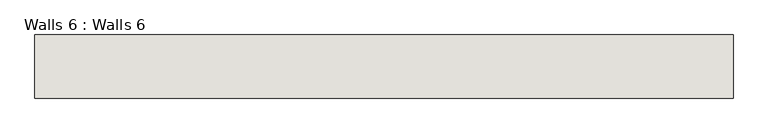
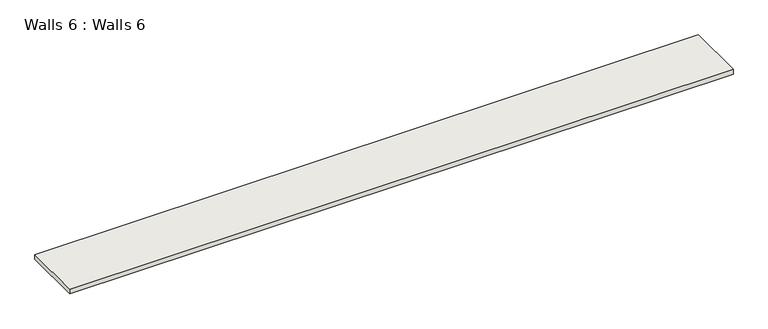
"""IFC4 building model written with IfcOpenShell, lengths in millimetres: wall geometry, Walls 6 : Walls 6."""

from ifc_helpers import new_model, si_unit, frame, origin, place, context, project, spatial, polyline, outline, extrude, source, transform, mapped, element, save


def walls_6_walls_6_8e6cdcdd(model_context):
    return source(origin(), model_context, "Body", "SweptSolid", [
        extrude(outline(polyline([(-2702.0878119, -3795.4929435), (-2702.0878119, -3420.8536983), (1438.1121881, -3420.8536983), (1438.1121881, -3795.4929435), (-2702.0878119, -3795.4929435)])), frame((0.0, 0.0, 3431.083015), z_axis=(0.0, 0.0, 1.0), x_axis=(1.0, 0.0, 0.0)), (0.0, 0.0, 1.0), 31.809103),
    ])


if __name__ == "__main__":
    model = new_model("IFC4")
    model_context = context("Model", 3, world=origin())
    ifc_project = project(units=[si_unit("LENGTHUNIT", "METRE", prefix="MILLI")], contexts=[model_context])
    site = spatial("IfcSite", under=ifc_project)
    building = spatial("IfcBuilding", under=site)
    placement = place(None, origin())
    walls_6_walls_6_shape = walls_6_walls_6_8e6cdcdd(model_context)
    element("IfcWall", 1, ObjectType="Walls 6 : Walls 6", at=placement, inside=building, context=model_context, shape_type="MappedRepresentation", body=[
        mapped(walls_6_walls_6_shape, transform((0.0, 0.0, 0.0), x_axis=(1.0, 0.0, 0.0), y_axis=(0.0, 1.0, 0.0), z_axis=(0.0, 0.0, 1.0))),
    ])
    save(model, "model.ifc")

# Revit data of these elements
# Element 1 (IfcWall, "Walls 6 : Walls 6")
#   Materials on its faces: "Default Wall"
# Materials
#   "Default Wall": colour RGB 80 80 80, transparency 0
